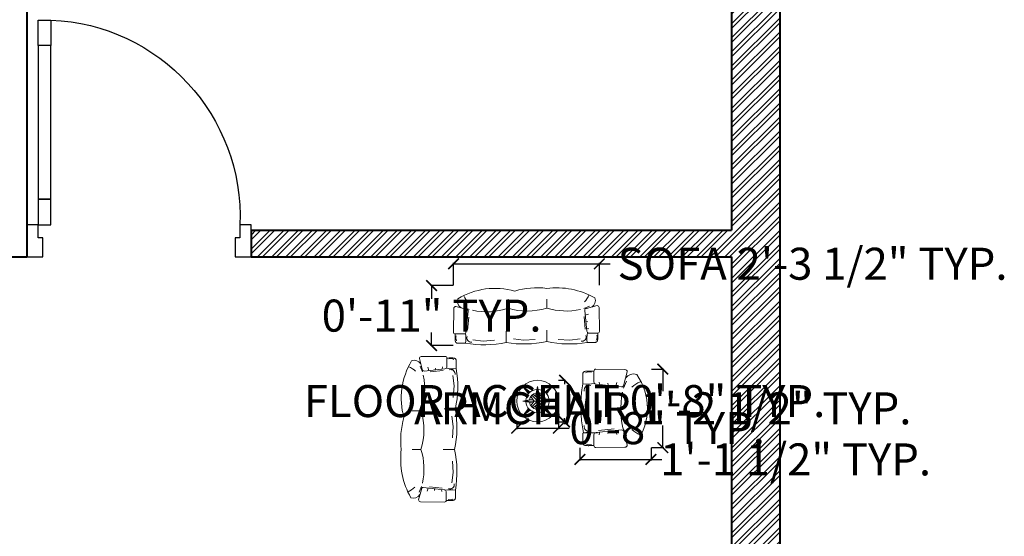
# Model space of a CAD drawing. Units: inches. Extents: x 528 to 2520, y -151 to 1354.
# Tile 36 of 41: x 2315 to 2499, y 635 to 731. Entities that reach past the tile are written whole.
import ezdxf

# ---------------------------------------------------------------- set-up
doc = ezdxf.new("R2010")
doc.units = ezdxf.units.IN
doc.header["$MEASUREMENT"] = 0
for name, color, linetype, lineweight in [('A-ANNO-DIMS', 2, 'Continuous', 18), ('A-Door', 150, 'Continuous', 25), ('A-ELEV-PROJ', 8, 'Continuous', 13), ('A-FURN', 8, 'Continuous', 18), ('A-WALL-PATT', 6, 'Continuous', 13), ('walls', 7, 'Continuous', 40)]:
    doc.layers.add(name, color=color, linetype=linetype, lineweight=lineweight)
doc.layers.add('NT', color=1, linetype='Continuous')
doc.styles.get("Standard").update_dxf_attribs({"font": 'arial.ttf'})
doc.dimstyles.get("Standard").update_dxf_attribs({"dimtxt": 6, "dimasz": 2, "dimexe": 0.18, "dimexo": 0.0625, "dimgap": 0.09, "dimtad": 0, "dimtih": 1, "dimtoh": 1, "dimdec": 1, "dimzin": 0, "dimdsep": 46, "dimlunit": 3, "dimtxsty": 'Standard', "dimblk": 'ARCHTICK', "dimcen": 0.09, "dimadec": 0, "dimazin": 0, "dimtfac": 1, "dimtdec": 1, "dimtofl": 0, "dimtmove": 0, "dimatfit": 3, "dimfxl": 1, "dimtolj": 1, "dimtzin": 0, "dimarcsym": 0})

# ---------------------------------------------------------------- blocks, each defined once
blk = doc.blocks.new('A$C7DB75F4D')
at = {"layer": 'A-Door'}
for points in [[(625, 740), (625, 660), (665, 660), (665, 740)], [(625, 180), (625, 660), (665, 660), (665, 180)], [(625, 100), (625, 180), (665, 180), (665, 100)], [(35, 100), (35, 60), (50, 60), (50, 50), (50, 0), (0, 0), (0, 100)], [(665, 100), (700, 100), (700, 0), (650, 0), (650, 50), (650, 60), (665, 60)]]:
    blk.add_lwpolyline(points, close=True, dxfattribs=at)
at = {"layer": 'NT'}
blk.add_arc((650, 125), 615.5, 92.3278, 182.3278, dxfattribs=at)
blk = doc.blocks.new('floor')
for p, q in [((-9.5, 11.5), (-18.9, 18.9)), ((-18.9, 18.9), (-10.6, 10.6)), ((-18.9, 18.9), (-11.6, 9.4)), ((0, 18.9), (-2.4, 6.1)), ((2.4, 6.1), (0, 18.9)), ((0, 18.9), (0, 2.1)), ((18.9, 18.9), (9.4, 11.5)), ((18.9, 18.9), (10.6, 10.6)), ((11.5, 9.4), (18.9, 18.9)), ((-6.1, 2.4), (-18.9, 0)), ((-18.9, 0), (-6.1, -2.4)), ((-18.9, 0), (-2.1, 0)), ((-8.7, 5.8), (-4.2, 0)), ((-7.4, 7.4), (-1.5, 1.5)), ((0, 4.2), (-5.8, 8.7)), ((5.8, 8.7), (0, 4.2)), ((7.4, 7.4), (1.5, 1.5)), ((2.1, 0), (18.9, 0)), ((4.2, 0), (8.7, 5.8)), ((18.9, 0), (6.1, 2.4)), ((6.1, -2.4), (18.9, 0)), ((-11.6, -9.5), (-18.9, -18.9)), ((-10.6, -10.6), (-18.9, -18.9)), ((-18.9, -18.9), (-9.5, -11.6)), ((-4.2, 0), (-8.7, -5.8)), ((-1.5, -1.5), (-7.4, -7.4)), ((-5.8, -8.7), (0, -4.2)), ((-2.4, -6.1), (0, -18.9)), ((0, -2.1), (0, -18.9)), ((0, -4.2), (5.8, -8.7)), ((0, -18.9), (2.4, -6.1)), ((1.5, -1.5), (7.4, -7.4)), ((8.7, -5.8), (4.2, 0)), ((9.4, -11.6), (18.9, -18.9)), ((10.6, -10.6), (18.9, -18.9)), ((18.9, -18.9), (11.5, -9.5))]:
    blk.add_line(p, q)
for radius in [26.7, 2.1]:
    blk.add_circle((0, 0), radius)
for radius, start, end in [(14.9, 92.8609, 177.1391), (14.9, 2.8609, 87.1391), (10.5, 98.7017, 171.2983), (10.5, 8.7017, 81.2983), (14.9, 182.8609, 267.1391), (10.5, 188.7017, 261.2983), (14.9, 272.8609, 357.1391), (10.5, 278.7017, 351.2983)]:
    blk.add_arc((0, 0), radius, start, end)
blk = doc.blocks.new('3-s')
for p, q in [((-3099.98, -914.27), (-3099.98, -918.75)), ((-3086.85, -913.54), (-3099.1, -913.37)), ((-3087.27, -919.9), (-3085.85, -914.54)), ((-3104.73, -915.45), (-3104.73, -919.55)), ((-3098.98, -919.75), (-3088.27, -920.9)), ((-3097.59, -919.77), (-3097.73, -918.83)), ((-3093.97, -920.17), (-3094.1, -919.37)), ((-3090.75, -920.58), (-3090.21, -918.96)), ((-3086.18, -918.42), (-3087.39, -921.38)), ((-3102.96, -923.27), (-3103.63, -928.52)), ((-3091.42, -921.25), (-3098, -920.58)), ((-3103.63, -928.52), (-3103.23, -934.44)), ((-3104.33, -940.39), (-3098.51, -940.39)), ((-3087.08, -940.39), (-3082.49, -940.39)), ((-3103.63, -952.27), (-3103.23, -946.35)), ((-3102.96, -957.52), (-3103.63, -952.27)), ((-3087.15, -960.23), (-3082.56, -960.23)), ((-3104.73, -961.23), (-3098.92, -961.23)), ((-3104.04, -973.11), (-3103.63, -967.19)), ((-3103.37, -978.36), (-3104.04, -973.11)), ((-3091.82, -980.37), (-3098.4, -981.05)), ((-3086.59, -983.2), (-3087.79, -980.24)), ((-3105.14, -986.18), (-3105.14, -982.07)), ((-3098, -981.85), (-3098.13, -982.8)), ((-3094.37, -981.45), (-3094.51, -982.26)), ((-3091.15, -981.05), (-3090.61, -982.66))]:
    blk.add_line(p, q)
for points in [[(-3099.98, -914.27), (-3100.65, -914.23), (-3101.21, -914.21), (-3101.68, -914.19), (-3102.07, -914.18), (-3102.4, -914.18), (-3102.68, -914.19), (-3102.91, -914.21), (-3103.11, -914.22), (-3103.29, -914.24), (-3103.46, -914.26), (-3103.62, -914.29), (-3103.76, -914.33), (-3103.89, -914.36), (-3104.01, -914.41), (-3104.12, -914.47), (-3104.23, -914.53), (-3104.33, -914.6), (-3104.43, -914.69), (-3104.51, -914.78), (-3104.58, -914.89), (-3104.65, -915.01), (-3104.69, -915.14), (-3104.72, -915.29), (-3104.73, -915.45)], [(-3100.39, -987.35), (-3101.05, -987.39), (-3101.61, -987.42), (-3102.08, -987.43), (-3102.48, -987.44), (-3102.81, -987.44), (-3103.08, -987.43), (-3103.31, -987.42), (-3103.51, -987.4), (-3103.7, -987.38), (-3103.87, -987.36), (-3104.02, -987.33), (-3104.16, -987.3), (-3104.29, -987.26), (-3104.41, -987.21), (-3104.53, -987.16), (-3104.63, -987.09), (-3104.73, -987.02), (-3104.83, -986.94), (-3104.91, -986.84), (-3104.99, -986.73), (-3105.05, -986.61), (-3105.1, -986.48), (-3105.13, -986.34), (-3105.14, -986.18)]]:
    blk.add_lwpolyline(points)
blk.add_lwpolyline([(-3087.67, -981.72), (-3086.25, -987.09, -0.414214), (-3087.25, -988.09), (-3099.51, -988.25, -0.464301), (-3100.39, -987.35), (-3100.39, -982.87, -0.414214), (-3099.39, -981.87), (-3088.67, -980.72, -0.414214)], format="xyb", close=True)
for centre, radius, start, end in [((-3101.91, -917.78), 3.27, 72.9324, 119.1125), ((-3099.16, -914.2), 0.826, 85.8896, 185.5116), ((-3086.85, -914.54), 1, 0, 90), ((-3051.57, -928.95), 53.99, 169.9808, 192.2408), ((-3102.44, -907.13), 12.63, 259.551, 282.5683), ((-3098.98, -918.75), 1, 180, 270), ((-3088.27, -919.9), 1, 270, 0), ((-3083.18, -919.47), 4.05, 71.0879, 146.7483), ((-3074.56, -931.19), 13.81, 115.1439, 132.7066), ((-3117.09, -935.46), 40.42, 352.9967, 29.3731), ((-3101.95, -922.43), 2.24, 70.9224, 187.7848), ((-3055.23, -930.36), 33.39, 167.467, 197.4804), ((-3051.57, -951.84), 53.99, 167.7592, 190.0192), ((-3055.23, -950.42), 33.39, 162.5196, 197.0763), ((-3117.09, -945.32), 40.42, 343.5213, 7.0033), ((-3055.63, -971.26), 33.39, 160.7021, 192.533), ((-3114.19, -966.81), 37.23, 329.0051, 15.6244), ((-3051.97, -972.68), 53.99, 167.7592, 190.0192), ((-3102.35, -979.2), 2.24, 172.2152, 289.0776), ((-3074.97, -970.43), 13.81, 227.2934, 244.8561), ((-3102.84, -994.5), 12.63, 77.4317, 100.449), ((-3083.58, -982.16), 4.05, 213.2517, 288.9121), ((-3102.31, -983.84), 3.27, 240.8875, 287.0676)]:
    blk.add_arc(centre, radius, start, end)
blk = doc.blocks.new('si-s')
for p, q in [((-3100.11, -942.03), (-3112.37, -941.87)), ((-3118, -943.94), (-3118, -948.05)), ((-3113.25, -942.77), (-3113.25, -947.25)), ((-3100.54, -948.4), (-3099.11, -943.03)), ((-3112.25, -948.25), (-3101.54, -949.4)), ((-3104.68, -949.75), (-3111.26, -949.07)), ((-3110.86, -948.27), (-3110.99, -947.32)), ((-3107.24, -948.67), (-3107.37, -947.86)), ((-3104.01, -949.07), (-3103.48, -947.46)), ((-3099.45, -946.92), (-3100.66, -949.88)), ((-3116.23, -951.76), (-3116.9, -957.01)), ((-3116.9, -957.01), (-3116.5, -962.93)), ((-3104.68, -967.23), (-3111.26, -967.9)), ((-3099.45, -970.06), (-3100.66, -967.1)), ((-3118, -973.03), (-3118, -968.93)), ((-3117.6, -968.89), (-3111.78, -968.89)), ((-3113.25, -974.21), (-3113.25, -969.73)), ((-3112.25, -968.73), (-3101.54, -967.58)), ((-3110.86, -968.71), (-3110.99, -969.65)), ((-3107.24, -968.31), (-3107.37, -969.11)), ((-3104.01, -967.9), (-3103.48, -969.52)), ((-3100.54, -968.58), (-3099.11, -973.94)), ((-3100.11, -974.94), (-3112.37, -975.11))]:
    blk.add_line(p, q)
for points in [[(-3113.25, -942.77), (-3113.92, -942.73), (-3114.48, -942.7), (-3114.95, -942.69), (-3115.34, -942.68), (-3115.67, -942.68), (-3115.94, -942.69), (-3116.18, -942.7), (-3116.38, -942.72), (-3116.56, -942.74), (-3116.73, -942.76), (-3116.88, -942.79), (-3117.03, -942.82), (-3117.16, -942.86), (-3117.28, -942.91), (-3117.39, -942.96), (-3117.5, -943.02), (-3117.6, -943.1), (-3117.69, -943.18), (-3117.78, -943.28), (-3117.85, -943.39), (-3117.91, -943.51), (-3117.96, -943.64), (-3117.99, -943.78), (-3118, -943.94)], [(-3113.25, -974.21), (-3113.92, -974.25), (-3114.48, -974.27), (-3114.95, -974.29), (-3115.34, -974.3), (-3115.67, -974.3), (-3115.94, -974.29), (-3116.18, -974.28), (-3116.38, -974.26), (-3116.56, -974.24), (-3116.73, -974.22), (-3116.88, -974.19), (-3117.03, -974.16), (-3117.16, -974.12), (-3117.28, -974.07), (-3117.39, -974.02), (-3117.5, -973.95), (-3117.6, -973.88), (-3117.69, -973.79), (-3117.78, -973.7), (-3117.85, -973.59), (-3117.91, -973.47), (-3117.96, -973.34), (-3117.99, -973.19), (-3118, -973.03)]]:
    blk.add_lwpolyline(points)
for centre, radius, start, end in [((-3112.43, -942.69), 0.826, 85.8896, 185.5116), ((-3100.11, -943.03), 1, 0, 90), ((-3115.18, -946.28), 3.27, 72.9324, 119.1125), ((-3096.45, -947.96), 4.05, 71.0879, 146.7483), ((-3115.55, -958.49), 24.96, 324.8902, 35.1098), ((-3064.84, -957.44), 53.99, 169.9808, 192.2408), ((-3115.71, -935.62), 12.63, 259.551, 282.5683), ((-3115.22, -950.92), 2.24, 70.9224, 187.7848), ((-3112.25, -947.25), 1, 180, 270), ((-3101.54, -948.4), 1, 270, 0), ((-3087.83, -959.69), 13.81, 115.1439, 132.7066), ((-3068.5, -958.86), 33.39, 167.467, 197.4804), ((-3115.22, -966.05), 2.24, 172.2152, 289.0776), ((-3087.83, -957.29), 13.81, 227.2934, 244.8561), ((-3115.71, -981.35), 12.63, 77.4317, 100.449), ((-3112.25, -969.73), 1, 90, 180), ((-3101.54, -968.58), 1, 0, 90), ((-3096.45, -969.01), 4.05, 213.2517, 288.9121), ((-3115.18, -970.7), 3.27, 240.8875, 287.0676), ((-3112.43, -974.29), 0.826, 174.4884, 274.1104), ((-3100.11, -973.94), 1, 270, 0)]:
    blk.add_arc(centre, radius, start, end)
blk = doc.blocks.new('_ArchTick')
at = {"color": 0, "linetype": 'ByBlock', "const_width": 0.15}
blk.add_lwpolyline([(-0.5, -0.5), (0.5, 0.5)], dxfattribs=at)
blk = doc.blocks.new('*D48')
at = {"layer": 'A-ANNO-DIMS', "color": 0, "lineweight": -2, "transparency": 16777216}
for p, q in [((2395.91, 681.62), (2395.91, 685.84)), ((2395.91, 685.66), (2423.24, 685.66)), ((2423.24, 681.62), (2423.24, 685.84)), ((2423.24, 685.66), (2425.24, 685.66))]:
    blk.add_line(p, q, dxfattribs=at)
at = {"layer": 'Defpoints', "color": 0, "transparency": 16777216}
for p in [(2423.24, 685.66), (2395.91, 681.56), (2423.24, 681.56)]:
    blk.add_point(p, dxfattribs=at)
at = {"layer": 'A-ANNO-DIMS', "color": 0, "lineweight": -2, "transparency": 16777216, "xscale": 2, "yscale": 2, "zscale": 2, "rotation": 180}
blk.add_blockref('_ArchTick', (2395.91, 685.66), dxfattribs=at)
at = {"layer": 'A-ANNO-DIMS', "color": 0, "lineweight": -2, "transparency": 16777216, "xscale": 2, "yscale": 2, "zscale": 2}
blk.add_blockref('_ArchTick', (2423.24, 685.66), dxfattribs=at)
at = {"layer": 'A-ANNO-DIMS', "color": 0, "transparency": 16777216, "insert": (2463.17, 685.66), "char_height": 6, "attachment_point": 5}
blk.add_mtext('\\A1;SOFA 2\'-3 1/2" TYP.', dxfattribs=at)
blk = doc.blocks.new('*D49')
at = {"layer": 'A-ANNO-DIMS', "color": 0, "lineweight": -2, "transparency": 16777216}
for p, q in [((2395.85, 681.56), (2391.63, 681.56)), ((2391.81, 681.56), (2391.81, 679.09)), ((2391.81, 670.32), (2391.81, 672.79)), ((2395.85, 670.32), (2391.63, 670.32))]:
    blk.add_line(p, q, dxfattribs=at)
at = {"layer": 'Defpoints', "color": 0, "transparency": 16777216}
for p in [(2391.81, 681.56), (2395.91, 681.56), (2395.91, 670.32)]:
    blk.add_point(p, dxfattribs=at)
at = {"layer": 'A-ANNO-DIMS', "color": 0, "lineweight": -2, "transparency": 16777216, "xscale": 2, "yscale": 2, "zscale": 2}
for p, rotation in [((2391.81, 681.56), 90), ((2391.81, 670.32), 270)]:
    blk.add_blockref('_ArchTick', p, dxfattribs=dict(at, rotation=rotation))
at = {"layer": 'A-ANNO-DIMS', "color": 0, "transparency": 16777216, "insert": (2391.81, 675.94), "char_height": 6, "attachment_point": 5}
blk.add_mtext('\\A1;0\'-11" TYP.', dxfattribs=at)
blk = doc.blocks.new('*D80')
at = {"layer": 'A-ANNO-DIMS', "color": 0, "lineweight": -2, "transparency": 16777216}
for p, q in [((2415.61, 663.82), (2416.9, 663.82)), ((2416.72, 663.82), (2416.72, 663.12)), ((2416.72, 656.02), (2416.72, 656.73)), ((2415.61, 656.02), (2416.9, 656.02))]:
    blk.add_line(p, q, dxfattribs=at)
at = {"layer": 'Defpoints', "color": 0, "transparency": 16777216}
for p in [(2415.55, 663.82), (2416.72, 663.82), (2415.55, 656.02)]:
    blk.add_point(p, dxfattribs=at)
at = {"layer": 'A-ANNO-DIMS', "color": 0, "lineweight": -2, "transparency": 16777216, "xscale": 2, "yscale": 2, "zscale": 2}
for p, rotation in [((2416.72, 663.82), 90), ((2416.72, 656.02), 270)]:
    blk.add_blockref('_ArchTick', p, dxfattribs=dict(at, rotation=rotation))
at = {"layer": 'A-ANNO-DIMS', "color": 0, "transparency": 16777216, "insert": (2416.72, 659.92), "char_height": 6, "attachment_point": 5}
blk.add_mtext('\\A1;FLOOR ACCENT 0\'-8" TYP.', dxfattribs=at)
blk = doc.blocks.new('*D81')
at = {"layer": 'A-ANNO-DIMS', "color": 0, "lineweight": -2, "transparency": 16777216}
for p, q in [((2407.75, 655.96), (2407.75, 654.67)), ((2407.75, 654.85), (2415.55, 654.85)), ((2415.55, 655.96), (2415.55, 654.67)), ((2415.55, 654.85), (2417.55, 654.85))]:
    blk.add_line(p, q, dxfattribs=at)
at = {"layer": 'Defpoints', "color": 0, "transparency": 16777216}
for p in [(2407.75, 656.02), (2415.55, 656.02), (2415.55, 654.85)]:
    blk.add_point(p, dxfattribs=at)
at = {"layer": 'A-ANNO-DIMS', "color": 0, "lineweight": -2, "transparency": 16777216, "xscale": 2, "yscale": 2, "zscale": 2, "rotation": 180}
blk.add_blockref('_ArchTick', (2407.75, 654.85), dxfattribs=at)
at = {"layer": 'A-ANNO-DIMS', "color": 0, "lineweight": -2, "transparency": 16777216, "xscale": 2, "yscale": 2, "zscale": 2}
blk.add_blockref('_ArchTick', (2415.55, 654.85), dxfattribs=at)
at = {"layer": 'A-ANNO-DIMS', "color": 0, "transparency": 16777216, "insert": (2435.93, 654.85), "char_height": 6, "attachment_point": 5}
blk.add_mtext('\\A1;0\'-8" TYP.', dxfattribs=at)
blk = doc.blocks.new('*D82')
at = {"layer": 'A-ANNO-DIMS', "color": 0, "lineweight": -2, "transparency": 16777216}
for p, q in [((2432.97, 665.92), (2435.29, 665.92)), ((2435.11, 665.92), (2435.11, 661.75)), ((2435.11, 651.2), (2435.11, 655.37)), ((2432.97, 651.2), (2435.29, 651.2))]:
    blk.add_line(p, q, dxfattribs=at)
at = {"layer": 'Defpoints', "color": 0, "transparency": 16777216}
for p in [(2432.91, 665.92), (2435.11, 665.92), (2432.91, 651.2)]:
    blk.add_point(p, dxfattribs=at)
at = {"layer": 'A-ANNO-DIMS', "color": 0, "lineweight": -2, "transparency": 16777216, "xscale": 2, "yscale": 2, "zscale": 2}
for p, rotation in [((2435.11, 665.92), 90), ((2435.11, 651.2), 270)]:
    blk.add_blockref('_ArchTick', p, dxfattribs=dict(at, rotation=rotation))
at = {"layer": 'A-ANNO-DIMS', "color": 0, "transparency": 16777216, "insert": (2435.11, 658.56), "char_height": 6, "attachment_point": 5}
blk.add_mtext('\\A1;ARMCHAIR 1\'-2 1/2" TYP.', dxfattribs=at)
blk = doc.blocks.new('*D83')
at = {"layer": 'A-ANNO-DIMS', "color": 0, "lineweight": -2, "transparency": 16777216}
for p, q in [((2419.58, 651.14), (2419.58, 648.81)), ((2432.91, 651.14), (2432.91, 648.81)), ((2419.58, 648.99), (2432.91, 648.99)), ((2432.91, 648.99), (2434.91, 648.99))]:
    blk.add_line(p, q, dxfattribs=at)
at = {"layer": 'Defpoints', "color": 0, "transparency": 16777216}
for p in [(2419.58, 651.2), (2432.91, 651.2), (2432.91, 648.99)]:
    blk.add_point(p, dxfattribs=at)
at = {"layer": 'A-ANNO-DIMS', "color": 0, "lineweight": -2, "transparency": 16777216, "xscale": 2, "yscale": 2, "zscale": 2, "rotation": 180}
blk.add_blockref('_ArchTick', (2419.58, 648.99), dxfattribs=at)
at = {"layer": 'A-ANNO-DIMS', "color": 0, "lineweight": -2, "transparency": 16777216, "xscale": 2, "yscale": 2, "zscale": 2}
blk.add_blockref('_ArchTick', (2432.91, 648.99), dxfattribs=at)
at = {"layer": 'A-ANNO-DIMS', "color": 0, "transparency": 16777216, "insert": (2459.99, 648.99), "char_height": 6, "attachment_point": 5}
blk.add_mtext('\\A1;1\'-1 1/2" TYP.', dxfattribs=at)

msp = doc.modelspace()

# ---------------------------------------------------------------- hatches: boundary and pattern name
at = {"layer": 'A-WALL-PATT'}
h = msp.add_hatch(dxfattribs=at)
h.set_pattern_fill('ANSI32', color=256, scale=5)
h.set_pattern_definition([(45, (1571.3155, -419.1643), (-1.3258252, 1.3258252), []), (45, (1572.1993, -419.1643), (-1.3258252, 1.3258252), [])])
h.paths.add_polyline_path([(2167.01, 744.69), (2158.01, 744.69), (2158.01, 549.94), (2169.56, 549.94), (2174.56, 549.94), (2174.56, 554.94), (2167.01, 554.94), (2167.01, 662.94), (2263.01, 662.94), (2263.01, 667.94), (2263.01, 686.94), (2269.01, 686.94), (2269.01, 691.94), (2258.01, 691.94), (2258.01, 667.94), (2167.01, 667.94)])
h.paths.add_polyline_path([(2260.02, 554.94), (2222.56, 554.94), (2222.56, 549.94), (2260.02, 549.94)])
h.paths.add_polyline_path([(2457.01, 752.2), (2448.01, 752.2), (2448.01, 691.94), (2358.01, 691.94), (2358.01, 686.94), (2448.01, 686.94), (2448.01, 554.94), (2358.01, 554.94), (2358.01, 549.94), (2448.01, 549.94), (2448.01, 405.94), (2406.01, 405.94), (2406.01, 396.94), (2457.01, 396.94)])
h.paths.add_polyline_path([(2457.01, 897.94), (2447.97, 897.94), (2447.97, 888.94), (2448.01, 888.94), (2448.01, 828.94), (2394.01, 828.94), (2394.01, 823.94), (2448.01, 823.94), (2448.01, 800.2), (2457.01, 800.2)])
h.paths.add_polyline_path([(2423.97, 897.94), (2359.01, 897.94), (2359.01, 828.94), (2355.58, 828.94), (2355.58, 823.94), (2364.01, 823.94), (2364.01, 829.94), (2364.01, 888.94), (2423.97, 888.94)])
h.paths.add_polyline_path([(2256.01, 897.94), (2191.01, 897.94), (2191.01, 888.94), (2251.01, 888.94), (2251.01, 828.94), (2251.01, 823.94), (2256.01, 823.94), (2256.01, 829.08)])
h.paths.add_polyline_path([(2167.01, 888.94), (2167.01, 897.94), (2158.01, 897.94), (2158.01, 792.69), (2167.01, 792.69), (2167.01, 823.94), (2221.01, 823.94), (2221.01, 828.94), (2167.01, 828.94)])
h.paths.add_polyline_path([(2316.01, 549.94), (2316.01, 554.94), (2296.02, 554.94), (2296.02, 549.94), (2311.01, 549.94), (2311.01, 455.12), (2316.01, 455.12)])
h.paths.add_polyline_path([(2311.01, 549.94), (2299.01, 549.94), (2299.01, 545.95), (2302.05, 545.95), (2302.05, 542.51), (2305.75, 542.51), (2305.75, 538.08), (2311.01, 538.08)], flags=17)
h.paths.add_polyline_path([(2358.01, 405.94), (2316.01, 405.94), (2316.01, 413.12), (2311.01, 413.12), (2311.01, 396.94), (2358.01, 396.94)])

# ---------------------------------------------------------------- linework, layer by layer
at = {"layer": 'A-ELEV-PROJ'}
msp.add_line((2457.01, 360.94), (2457.01, 897.94), dxfattribs=at)
at = {"layer": 'walls'}
for p, q in [((2457.01, 897.94), (2457.01, 396.94)), ((2316.01, 823.94), (2316.01, 691.94)), ((2448.01, 823.94), (2448.01, 691.94)), ((2316.01, 691.94), (2316.01, 686.94)), ((2358.01, 691.94), (2448.01, 691.94)), ((2358.01, 691.94), (2358.01, 686.94)), ((2311.01, 686.94), (2316.01, 686.94)), ((2358.01, 686.94), (2448.01, 686.94)), ((2448.01, 686.94), (2448.01, 554.94))]:
    msp.add_line(p, q, dxfattribs=at)

# ---------------------------------------------------------------- block references
at = {"layer": 'A-Door', "xscale": -0.0600000000000059, "yscale": 0.0600000000000059, "zscale": 0.0600000000000059}
msp.add_blockref('A$C7DB75F4D', (2358.01, 686.94), dxfattribs=at)
at = {"layer": 'A-FURN'}
for p, xscale, yscale, zscale, rotation in [((2756.45, 1803.59), -0.3648213827119744, 0.3648213827119744, 0.3648213827119362, 270), ((1263.59, 307.77), 0.3648213827118212, 0.3648213827118212, 0.3648213827118212, 180)]:
    msp.add_blockref('3-s', p, dxfattribs=dict(at, xscale=xscale, yscale=yscale, zscale=zscale, rotation=rotation))
for name, p, xscale, yscale, zscale in [('si-s', (3799.06, 1082.45), 0.4422535540881025, 0.4422535540881025, 0.4422535540881025), ('floor', (2411.65, 659.92, -157.77), 0.1459285530847694, 0.1459285530847694, 0.1459285530847694)]:
    msp.add_blockref(name, p, dxfattribs=dict(at, xscale=xscale, yscale=yscale, zscale=zscale))

# ---------------------------------------------------------------- dimensions: what is measured, and where the dimension line sits
at = {"layer": 'A-ANNO-DIMS'}
for base, p1, p2, text, picture, middle in [((2423.24, 685.66), (2395.91, 681.56), (2423.24, 681.56), 'SOFA <> TYP.', '*D48', (2463.17, 685.66)), ((2415.55, 654.85), (2407.75, 656.02), (2415.55, 656.02), '<> TYP.', '*D81', (2435.93, 654.85)), ((2432.91, 648.99), (2419.58, 651.2), (2432.91, 651.2), '<> TYP.', '*D83', (2459.99, 648.99))]:
    dim = msp.add_linear_dim(base=base, p1=p1, p2=p2, text=text, dimstyle='Standard', override={"dimdec": 1, "dimlfac": 1, "dimrnd": 0, "dimzin": 1, "dimdsep": 46, "dimlunit": 4, "dimfrac": 2}, dxfattribs=at)
    dim.commit()
    dim.dimension.update_dxf_attribs({"geometry": picture, "text_midpoint": middle})
for base, p1, p2, text, picture, middle in [((2391.81, 681.56), (2395.91, 670.32), (2395.91, 681.56), '<> TYP.', '*D49', (2391.81, 675.94)), ((2416.72, 663.82), (2415.55, 656.02), (2415.55, 663.82), 'FLOOR ACCENT <> TYP.', '*D80', (2416.72, 659.92)), ((2435.11, 665.92), (2432.91, 651.2), (2432.91, 665.92), 'ARMCHAIR <> TYP.', '*D82', (2435.11, 658.56))]:
    dim = msp.add_linear_dim(base=base, p1=p1, p2=p2, angle=90, text=text, dimstyle='Standard', override={"dimdec": 1, "dimlfac": 1, "dimrnd": 0, "dimzin": 1, "dimdsep": 46, "dimlunit": 4, "dimfrac": 2}, dxfattribs=at)
    dim.commit()
    dim.dimension.update_dxf_attribs({"geometry": picture, "text_midpoint": middle})

doc.saveas('drawing.dxf')
